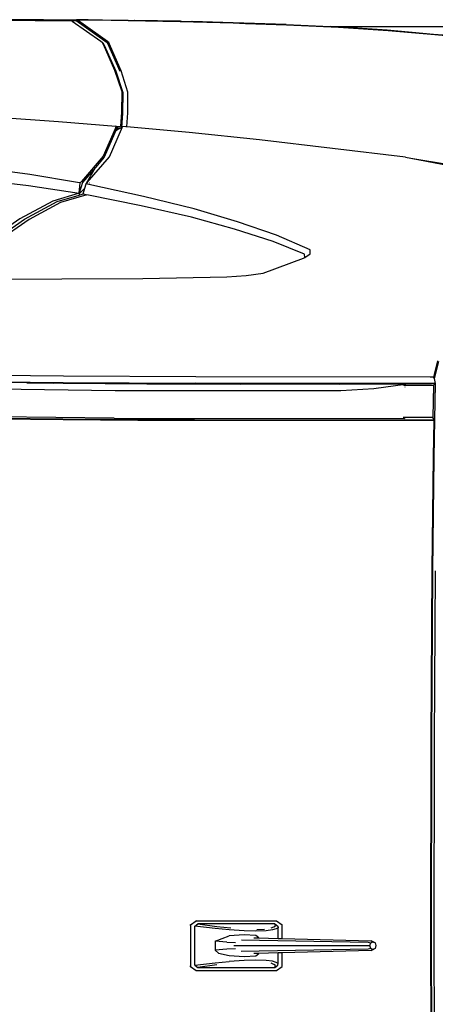
# Model space of a CAD drawing. Units: inches. Extents: x 22042254 to 25404563, y 17568978 to 17626777.
# Tile 17 of 45: x 22042342.6037 to 22042342.8522, y 17568978.1821 to 17568978.7711. Entities that reach past the tile are written whole.
import ezdxf

# ---------------------------------------------------------------- set-up
doc = ezdxf.new("R2010")
doc.units = ezdxf.units.IN
doc.header["$MEASUREMENT"] = 0
doc.layers.add('A-SITE-VEHI', color=8, linetype='Continuous', lineweight=18)
doc.layers.add('Edges', color=250, linetype='Continuous')

# ---------------------------------------------------------------- blocks, each defined once
blk = doc.blocks.new('Nissan Qashqai pl')
at = {"layer": 'Edges'}
for p, q in [((11.05474, 11.92208), (11.05507, 12.12031)), ((11.05537, 11.92208), (11.05571, 12.1202)), ((11.0586, 12.11975), (11.05827, 11.92208)), ((10.8228, 11.94208), (10.82239, 11.94208)), ((10.8228, 11.94208), (10.82834, 11.94608)), ((10.8228, 11.90208), (10.8228, 11.94208)), ((10.82696, 11.94083), (10.83007, 11.94308)), ((10.82696, 11.94083), (10.82696, 11.90333)), ((10.82696, 11.94083), (10.84666, 11.93861)), ((10.82794, 11.94608), (10.82834, 11.94608)), ((10.82834, 11.94608), (10.90603, 11.94608)), ((10.84833, 11.9406), (10.83007, 11.94308)), ((10.83007, 11.94308), (10.9043, 11.94308)), ((10.90348, 11.94026), (10.90076, 11.93914)), ((10.90503, 11.94137), (10.90348, 11.94026)), ((10.9043, 11.94308), (10.90741, 11.94083)), ((10.9043, 11.94308), (10.90503, 11.94137)), ((10.90744, 11.9393), (10.90565, 11.93837)), ((10.90603, 11.94608), (10.91157, 11.94208)), ((10.90741, 11.94083), (10.90744, 11.9393)), ((10.90744, 11.9393), (10.90744, 11.92915)), ((10.91157, 11.94208), (10.91157, 11.92904)), ((10.84666, 11.93861), (10.86027, 11.93735)), ((10.85007, 11.92947), (10.86027, 11.93157)), ((10.8746, 11.93634), (10.86027, 11.93735)), ((10.86027, 11.93157), (10.8746, 11.93265)), ((10.88611, 11.93611), (10.8746, 11.93634)), ((10.8746, 11.93265), (10.88611, 11.93193)), ((10.889, 11.92962), (10.88395, 11.92975)), ((10.89593, 11.93645), (10.88611, 11.93611)), ((10.88611, 11.93193), (10.889, 11.92962)), ((10.90744, 11.92915), (10.889, 11.92962)), ((10.90215, 11.93722), (10.89593, 11.93645)), ((10.90565, 11.93837), (10.90215, 11.93722)), ((10.84666, 11.92634), (10.85007, 11.92947)), ((10.84666, 11.91782), (10.84666, 11.92634)), ((10.85787, 11.92547), (10.84666, 11.92634)), ((10.86624, 11.92503), (10.85787, 11.92547)), ((10.86474, 11.92208), (10.99603, 11.92208)), ((10.99456, 11.92544), (10.87195, 11.92764)), ((10.91157, 11.92904), (10.90744, 11.92915)), ((10.99731, 11.92683), (10.91157, 11.92904)), ((10.99691, 11.92468), (10.99456, 11.92544)), ((10.99691, 11.92468), (10.99603, 11.92208)), ((10.99603, 11.92208), (10.99691, 11.91949)), ((10.99903, 11.92575), (10.99691, 11.92468)), ((10.99731, 11.92683), (11.00007, 11.92544)), ((10.99903, 11.92575), (10.99731, 11.92683)), ((11.00116, 11.92468), (10.99903, 11.92575)), ((11.00116, 11.92468), (11.00007, 11.92544)), ((11.00204, 11.92208), (11.00116, 11.92468)), ((11.00116, 11.91949), (11.00204, 11.92208)), ((11.05507, 11.72385), (11.05474, 11.92208)), ((11.05571, 11.72396), (11.05537, 11.92208)), ((11.05827, 11.92208), (11.0586, 11.72441)), ((10.85787, 11.91869), (10.84666, 11.91782)), ((10.84666, 11.91782), (10.86027, 11.91259)), ((10.85787, 11.91869), (10.86624, 11.91913)), ((10.8746, 11.91151), (10.86027, 11.91259)), ((10.87225, 11.91653), (10.99456, 11.91872)), ((10.88611, 11.91223), (10.8746, 11.91151)), ((10.88395, 11.91441), (10.889, 11.91454)), ((10.889, 11.91454), (10.88611, 11.91223)), ((10.889, 11.91454), (10.90744, 11.91502)), ((10.90744, 11.91502), (10.91157, 11.91512)), ((10.90744, 11.91502), (10.90744, 11.90486)), ((10.91157, 11.91512), (10.99731, 11.91733)), ((10.91157, 11.91512), (10.91157, 11.90208)), ((10.99456, 11.91872), (10.99691, 11.91949)), ((10.99691, 11.91949), (10.99903, 11.91841)), ((11.00007, 11.91872), (10.99731, 11.91733)), ((10.99731, 11.91733), (10.99903, 11.91841)), ((10.99903, 11.91841), (10.99963, 11.91871)), ((10.99963, 11.91871), (11.00116, 11.91949)), ((11.00007, 11.91872), (10.99963, 11.91871)), ((11.00116, 11.91949), (11.00007, 11.91872)), ((10.82239, 11.90208), (10.8228, 11.90208)), ((10.8228, 11.90208), (10.82834, 11.89808)), ((10.84666, 11.90555), (10.82696, 11.90333)), ((10.82696, 11.90333), (10.83007, 11.90108)), ((10.83007, 11.90108), (10.84833, 11.90356)), ((10.9043, 11.90108), (10.83007, 11.90108)), ((10.86027, 11.90681), (10.84666, 11.90555)), ((10.84833, 11.90356), (10.86193, 11.905)), ((10.8746, 11.90782), (10.86027, 11.90681)), ((10.88611, 11.90805), (10.8746, 11.90782)), ((10.89593, 11.90771), (10.88611, 11.90805)), ((10.88709, 11.90634), (10.89442, 11.90601)), ((10.90215, 11.90694), (10.89593, 11.90771)), ((10.90076, 11.90502), (10.90348, 11.9039)), ((10.90565, 11.90579), (10.90215, 11.90694)), ((10.90348, 11.9039), (10.90503, 11.90279)), ((10.9043, 11.90108), (10.90741, 11.90333)), ((10.90503, 11.90279), (10.9043, 11.90108)), ((10.90744, 11.90486), (10.90565, 11.90579)), ((10.90603, 11.89808), (10.91157, 11.90208)), ((10.90741, 11.90333), (10.90744, 11.90486)), ((10.90741, 11.90333), (10.90741, 11.90484)), ((10.82834, 11.89808), (10.82794, 11.89808)), ((10.82834, 11.89808), (10.90603, 11.89808)), ((11.05596, 11.55904), (11.05507, 11.72385)), ((11.0566, 11.5593), (11.05571, 11.72396)), ((11.0586, 11.72441), (11.05947, 11.55994)), ((11.05722, 11.44991), (11.05596, 11.55904)), ((11.05785, 11.45038), (11.0566, 11.5593)), ((11.05789, 11.4146), (11.05722, 11.44991)), ((11.05854, 11.41419), (11.05785, 11.45038)), ((10.69961, 11.41337), (10.55607, 11.41187)), ((10.5563, 11.41232), (10.69989, 11.41381)), ((10.7493, 11.41253), (10.62233, 11.41086)), ((10.77221, 11.41378), (10.69961, 11.41337)), ((10.69989, 11.41381), (10.77221, 11.4142)), ((10.7493, 11.41253), (11.02943, 11.41262)), ((10.77221, 11.4142), (10.78885, 11.41429)), ((10.77221, 11.4142), (10.77221, 11.41378)), ((10.78885, 11.41387), (10.77221, 11.41378)), ((10.78885, 11.41429), (10.79225, 11.41431)), ((10.78885, 11.41387), (10.78885, 11.41429)), ((10.79225, 11.41389), (10.78885, 11.41387)), ((10.79225, 11.41431), (10.79328, 11.41432)), ((10.79225, 11.41389), (10.79225, 11.41431)), ((10.79328, 11.4139), (10.79225, 11.41389)), ((10.79328, 11.41432), (10.82704, 11.4145)), ((10.79328, 11.4139), (10.79328, 11.41432)), ((10.82673, 11.41408), (10.79328, 11.4139)), ((10.82673, 11.41408), (11.05854, 11.41419)), ((10.82704, 11.4145), (11.05789, 11.4146)), ((11.02945, 11.41183), (11.02814, 11.41183)), ((11.02944, 11.41252), (11.02943, 11.41262)), ((11.05683, 11.41184), (11.02945, 11.41183)), ((11.02945, 11.41162), (11.02945, 11.41183)), ((11.05854, 11.41419), (11.05683, 11.41184)), ((11.05743, 11.38044), (11.05683, 11.41184)), ((11.05854, 11.41419), (11.05789, 11.4146)), ((11.05921, 11.37886), (11.05854, 11.41419)), ((10.55662, 11.37645), (10.69998, 11.37799)), ((10.6649, 11.37825), (10.55757, 11.37665)), ((10.6649, 11.37825), (10.58658, 11.37719)), ((10.62366, 11.38388), (10.75022, 11.38554)), ((10.69078, 11.37855), (10.6649, 11.37825)), ((10.6649, 11.37825), (10.67717, 11.37844)), ((10.69658, 11.37873), (10.67717, 11.37844)), ((10.67717, 11.37844), (10.69078, 11.37855)), ((10.69913, 11.37864), (10.69078, 11.37855)), ((10.71439, 11.37882), (10.69658, 11.37873)), ((10.69986, 11.37862), (10.69913, 11.37864)), ((10.69986, 11.37862), (10.78083, 11.37927)), ((10.71439, 11.37882), (10.69986, 11.37862)), ((10.69998, 11.37799), (10.82786, 11.37874)), ((10.72388, 11.37887), (10.71439, 11.37882)), ((10.72479, 11.37891), (10.72388, 11.37887)), ((10.78083, 11.37927), (10.72479, 11.37891)), ((10.75022, 11.38554), (10.96805, 11.38566)), ((10.78083, 11.37927), (10.8711, 11.37956)), ((10.94306, 11.3796), (10.82786, 11.37874)), ((10.82786, 11.37874), (11.05524, 11.37886)), ((10.96142, 11.37881), (10.82786, 11.37874)), ((10.89604, 11.37957), (10.8711, 11.37956)), ((10.90974, 11.3796), (10.89604, 11.37957)), ((10.94306, 11.3796), (10.90974, 11.3796)), ((10.94785, 11.37963), (10.94306, 11.3796)), ((10.9491, 11.37964), (10.94785, 11.37963)), ((10.96679, 11.37961), (10.9491, 11.37964)), ((10.96142, 11.37881), (10.96679, 11.37961)), ((10.97113, 11.37881), (10.96142, 11.37881)), ((10.96679, 11.37961), (10.96696, 11.37964)), ((10.97653, 11.37962), (10.96696, 11.37964)), ((10.96805, 11.38566), (10.99996, 11.38365)), ((10.97653, 11.37962), (10.97113, 11.37881)), ((10.97664, 11.37882), (10.97113, 11.37881)), ((10.98248, 11.37964), (10.97653, 11.37962)), ((10.97653, 11.37962), (10.97664, 11.37882)), ((11.05921, 11.37886), (10.97664, 11.37882)), ((11.03007, 11.37965), (10.98248, 11.37964)), ((10.99996, 11.38365), (11.03007, 11.37965)), ((11.02869, 11.38043), (11.03005, 11.38043)), ((11.03005, 11.38025), (11.02923, 11.38024)), ((11.03002, 11.38217), (11.03001, 11.38239)), ((11.03005, 11.38043), (11.05544, 11.38044)), ((11.05544, 11.38044), (11.03005, 11.38025)), ((11.03005, 11.38025), (11.03005, 11.38043)), ((11.03007, 11.37965), (11.03005, 11.38025)), ((11.05544, 11.38044), (11.05743, 11.38044)), ((11.05921, 11.37886), (11.05743, 11.38044)), ((11.05822, 11.37418), (11.05921, 11.37886)), ((10.7004, 11.37196), (10.55723, 11.37045)), ((10.82794, 11.37265), (10.7004, 11.37196)), ((11.05437, 11.37279), (10.82794, 11.37265)), ((11.05754, 11.37277), (11.05437, 11.37279)), ((11.05822, 11.37418), (11.05754, 11.37277)), ((11.05807, 11.37037), (11.05754, 11.37277)), ((11.06139, 11.35691), (11.05807, 11.37037)), ((11.06236, 11.3576), (11.05822, 11.37418)), ((10.58925, 11.27827), (10.69879, 11.27793)), ((10.69879, 11.27793), (10.77686, 11.27742)), ((10.77686, 11.27742), (10.85804, 11.27587)), ((10.85804, 11.27587), (10.87661, 11.27449)), ((10.87661, 11.27449), (10.89318, 11.27219)), ((10.89318, 11.27219), (10.932, 11.25799)), ((10.932, 11.25799), (10.93345, 11.25704)), ((10.93345, 11.25704), (10.93299, 11.25409)), ((10.93345, 11.25704), (10.93862, 11.25365)), ((10.65826, 11.2197), (10.62146, 11.24557)), ((10.62607, 11.24576), (10.6627, 11.22001)), ((10.6671, 11.22032), (10.63062, 11.24593)), ((10.93299, 11.25409), (10.90264, 11.24169)), ((10.9384, 11.24966), (10.90591, 11.23547)), ((10.93862, 11.25365), (10.9384, 11.24966)), ((10.90264, 11.24169), (10.86528, 11.22973)), ((10.90591, 11.23547), (10.86821, 11.22258)), ((10.86528, 11.22973), (10.82385, 11.21811)), ((10.69003, 11.20277), (10.65826, 11.2197)), ((10.6627, 11.22001), (10.6943, 11.20317)), ((10.69755, 11.20409), (10.6671, 11.22032)), ((10.82385, 11.21811), (10.77536, 11.20713)), ((10.86821, 11.22258), (10.82645, 11.21003)), ((10.77536, 11.20713), (10.72279, 11.1965)), ((10.82645, 11.21003), (10.77763, 11.19817)), ((10.71545, 11.19515), (10.69003, 11.20277)), ((10.6943, 11.20317), (10.71545, 11.19687)), ((10.72279, 11.1965), (10.69755, 11.20409)), ((10.77763, 11.19817), (10.72473, 11.18666)), ((10.61435, 11.18131), (10.66642, 11.18754)), ((10.66642, 11.18754), (10.71545, 11.19515)), ((10.71545, 11.1957), (10.71545, 11.19687)), ((10.71545, 11.19687), (10.71925, 11.19574)), ((10.72089, 11.19018), (10.71545, 11.1957)), ((10.71545, 11.19515), (10.71545, 11.1957)), ((10.71859, 11.18483), (10.71545, 11.19515)), ((10.71545, 11.19515), (10.71653, 11.1851)), ((10.71925, 11.19574), (10.72279, 11.1965)), ((10.71925, 11.19574), (10.72089, 11.19018)), ((10.72089, 11.19018), (10.7221, 11.18607)), ((10.71369, 11.18463), (10.6678, 11.17696)), ((10.71653, 11.1851), (10.71369, 11.18463)), ((10.71766, 11.18379), (10.71653, 11.1851)), ((10.73867, 11.15929), (10.71766, 11.18379)), ((10.73119, 11.17009), (10.71859, 11.18483)), ((10.7221, 11.18607), (10.72224, 11.1859)), ((10.7222, 11.18605), (10.7221, 11.18607)), ((10.72473, 11.18666), (10.7222, 11.18605)), ((10.7222, 11.18605), (10.72224, 11.1859)), ((10.72224, 11.1859), (10.72325, 11.18477)), ((10.72224, 11.1859), (10.72238, 11.18545)), ((10.72238, 11.18545), (10.73119, 11.17009)), ((10.72325, 11.18477), (10.72282, 11.18593)), ((10.72325, 11.18477), (10.74486, 11.15985)), ((10.72567, 11.18531), (10.72556, 11.18542)), ((11.03575, 11.16129), (11.1598, 11.18473)), ((10.6678, 11.17696), (10.61519, 11.17018)), ((10.73966, 11.16018), (10.73119, 11.17009)), ((11.04919, 11.16347), (11.13359, 11.17719)), ((10.75013, 11.13275), (10.73867, 11.15929)), ((10.75073, 11.1344), (10.73966, 11.16018)), ((10.74486, 11.15985), (10.75628, 11.13325)), ((11.03041, 11.16033), (10.88962, 11.14337)), ((11.03041, 11.16033), (11.03575, 11.16129)), ((11.03575, 11.16129), (11.04905, 11.16345)), ((11.04919, 11.16347), (11.04905, 11.16345)), ((10.88962, 11.14337), (10.82176, 11.13649)), ((10.75069, 11.13095), (10.75013, 11.13275)), ((10.75097, 11.13097), (10.75069, 11.13095)), ((10.75092, 11.13018), (10.75069, 11.13095)), ((10.75111, 11.13351), (10.75073, 11.1344)), ((10.75073, 11.1344), (10.75244, 11.13354)), ((10.75224, 11.13107), (10.75092, 11.13018)), ((10.75161, 11.13102), (10.75092, 11.13018)), ((10.75189, 11.13136), (10.75111, 11.13351)), ((10.75189, 11.13136), (10.75161, 11.13102)), ((10.75224, 11.13107), (10.75161, 11.13102)), ((10.75256, 11.13175), (10.75189, 11.13136)), ((10.75535, 11.13074), (10.75224, 11.13107)), ((10.75244, 11.13354), (10.75256, 11.13175)), ((10.75244, 11.13354), (10.75565, 11.13194)), ((10.75322, 11.13213), (10.75256, 11.13175)), ((10.75256, 11.13175), (10.75259, 11.13145)), ((10.75565, 11.13194), (10.75322, 11.13213)), ((10.75627, 11.1169), (10.75535, 11.13074)), ((10.75565, 11.13194), (10.75612, 11.1317)), ((10.75631, 11.13154), (10.75612, 11.1317)), ((10.75612, 11.1317), (10.75629, 11.13169)), ((10.75628, 11.13189), (10.75614, 11.1319)), ((10.75628, 11.13325), (10.75689, 11.13167)), ((10.75629, 11.13169), (10.75628, 11.13189)), ((10.75629, 11.13169), (10.75689, 11.13167)), ((10.7569, 11.13164), (10.75629, 11.13169)), ((10.75631, 11.13154), (10.75629, 11.13169)), ((10.75723, 11.11783), (10.75631, 11.13154)), ((10.75727, 11.1307), (10.75631, 11.13154)), ((10.75689, 11.13167), (10.7569, 11.13164)), ((10.7569, 11.13164), (10.75727, 11.1307)), ((10.76042, 11.13099), (10.75727, 11.1307)), ((10.76145, 11.13107), (10.76042, 11.13099)), ((10.82176, 11.13649), (10.76145, 11.13107)), ((10.76145, 11.13107), (10.76229, 11.1173)), ((10.63183, 11.12133), (10.69546, 11.12574)), ((10.69546, 11.12574), (10.75092, 11.13018)), ((10.75648, 11.09691), (10.75627, 11.1169)), ((10.75747, 11.09792), (10.75723, 11.11783)), ((10.76229, 11.1173), (10.76258, 11.09741)), ((10.74965, 11.07628), (10.75648, 11.09691)), ((10.7507, 11.07729), (10.75747, 11.09792)), ((10.76258, 11.09741), (10.75592, 11.07672)), ((10.73846, 11.051), (10.74965, 11.07628)), ((10.73956, 11.05193), (10.7507, 11.07729)), ((10.75486, 11.07758), (10.74298, 11.05028)), ((10.75592, 11.07672), (10.74477, 11.05114)), ((10.70875, 11.02887), (10.7363, 11.0483)), ((10.74241, 11.04987), (10.71254, 11.02855)), ((10.74291, 11.04852), (10.7148, 11.02842)), ((10.7363, 11.0483), (10.73758, 11.04917)), ((10.73869, 11.05016), (10.73758, 11.04917)), ((10.73758, 11.04917), (10.73776, 11.04954)), ((10.73776, 11.04954), (10.73846, 11.051)), ((10.73776, 11.04954), (10.73792, 11.04965)), ((10.73869, 11.05016), (10.73956, 11.05193)), ((10.74241, 11.04987), (10.74298, 11.05028)), ((10.74324, 11.04877), (10.74291, 11.04852)), ((10.74292, 11.04876), (10.74324, 11.04877)), ((10.74404, 11.04936), (10.74324, 11.04877)), ((10.74477, 11.05114), (10.74404, 11.04936)), ((11.01272, 11.03746), (10.9649, 11.03441)), ((10.9657, 11.03466), (11.01381, 11.03772)), ((11.05762, 11.04159), (11.01272, 11.03746)), ((11.01381, 11.03772), (11.05899, 11.04188)), ((11.07977, 11.04339), (11.05762, 11.04159)), ((11.05899, 11.04188), (11.07681, 11.04337)), ((10.61514, 11.02827), (10.66445, 11.02801)), ((10.66511, 11.02743), (10.61756, 11.02773)), ((10.66445, 11.02801), (10.7078, 11.02821)), ((10.67702, 11.02746), (10.66511, 11.02743)), ((10.70817, 11.02853), (10.67289, 11.02845)), ((10.68004, 11.02743), (10.67702, 11.02746)), ((10.68094, 11.02743), (10.68004, 11.02743)), ((10.68094, 11.02743), (10.71276, 11.02755)), ((10.7078, 11.02821), (10.70826, 11.02853)), ((10.70817, 11.02853), (10.7078, 11.02821)), ((10.70855, 11.02887), (10.70817, 11.02853)), ((10.70826, 11.02853), (10.70817, 11.02853)), ((10.70826, 11.02853), (10.70875, 11.02887)), ((10.71254, 11.02855), (10.70826, 11.02853)), ((10.71464, 11.02857), (10.71254, 11.02855)), ((10.71254, 11.02855), (10.71391, 11.02779)), ((10.71338, 11.02755), (10.71276, 11.02755)), ((10.76246, 11.02806), (10.71338, 11.02755)), ((10.72402, 11.02755), (10.71338, 11.02755)), ((10.7148, 11.02842), (10.71391, 11.02779)), ((10.76281, 11.02832), (10.71391, 11.02779)), ((10.72402, 11.02755), (10.76848, 11.02806)), ((10.76281, 11.02806), (10.76246, 11.02806)), ((10.76281, 11.02832), (10.81307, 11.02924)), ((10.76281, 11.02806), (10.81313, 11.029)), ((10.76883, 11.02806), (10.76848, 11.02806)), ((10.81313, 11.029), (10.76883, 11.02806)), ((10.81307, 11.02924), (10.86443, 11.03061)), ((10.81319, 11.029), (10.81313, 11.029)), ((10.81319, 11.029), (10.81393, 11.02902)), ((10.81418, 11.029), (10.81393, 11.02902)), ((10.81424, 11.029), (10.81418, 11.029)), ((10.81424, 11.029), (10.82415, 11.02929)), ((10.82419, 11.02929), (10.82415, 11.02929)), ((10.82464, 11.02931), (10.82419, 11.02929)), ((10.8642, 11.03037), (10.82464, 11.02931)), ((10.91525, 11.03213), (10.8642, 11.03037)), ((10.86421, 11.03053), (10.8759, 11.031)), ((10.86443, 11.03061), (10.8759, 11.031)), ((10.8759, 11.031), (10.91576, 11.03237)), ((10.91525, 11.03213), (10.95773, 11.03408)), ((10.91576, 11.03237), (10.9657, 11.03466)), ((10.9649, 11.03441), (10.95773, 11.03408)), ((10.95773, 11.03408), (11.12828, 11.03408))]:
    blk.add_line(p, q, dxfattribs=at)
blk = doc.blocks.new('CAR')
blk.add_blockref('Nissan Qashqai pl', (-9.74328, -11.91512))

msp = doc.modelspace()

# ---------------------------------------------------------------- block references
at = {"layer": 'A-SITE-VEHI', "xscale": -0.6191396643141144, "yscale": 0.6191396643141144, "zscale": 0.6191396643141144, "rotation": 180}
msp.add_blockref('CAR', (22042342.03736, 17568978.22147), dxfattribs=at)

doc.saveas('drawing.dxf')
